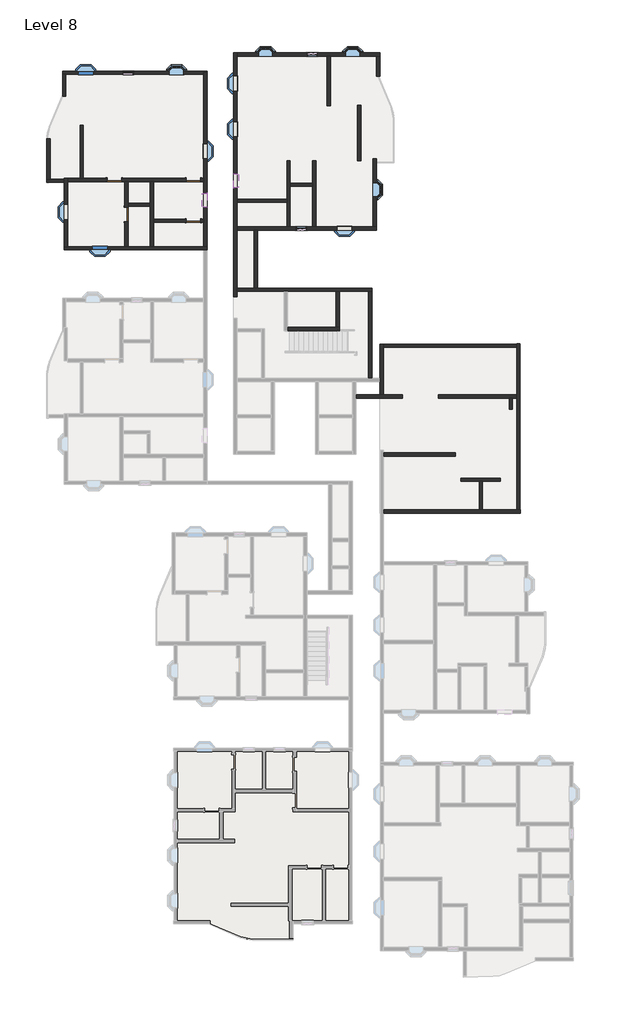
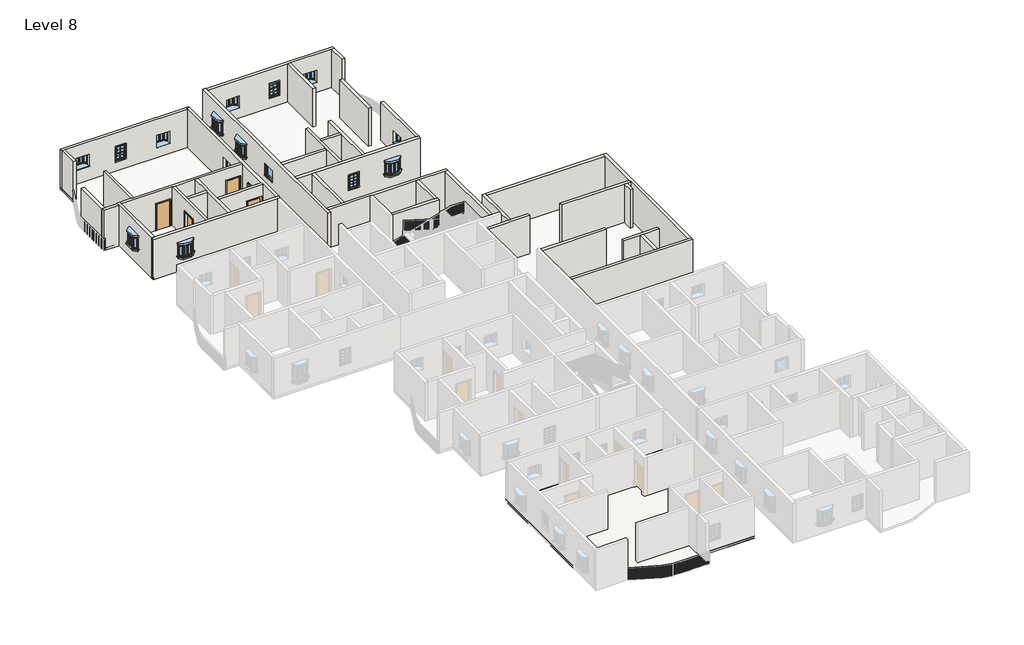
# One storey, part 4 of 14: 39 walls, 16 windows, 4 doors, 2 roofs.
"""IFC4 building model written with IfcOpenShell, lengths in millimetres."""

from ifc_helpers import new_model, si_unit, point, frame, frame_2d, origin, place, context, project, spatial, polyline, circle_curve, trimmed, segment, composite_curve, outline, extrude, faceted_brep, transform, mapped, element, save
from components import door_719f80de, window_910x910mm_67ef725a, window_8debb0fa, windows_sgl_w_glazing_bars_910x910mm_256712d0

model = new_model("IFC4")

# Units and contexts
model_context = context("Model", 3, world=origin())
ifc_project = project(units=[si_unit("LENGTHUNIT", "METRE", prefix="MILLI")], contexts=[model_context])

# Site, building, storey
site = spatial("IfcSite", under=ifc_project)
building = spatial("IfcBuilding", under=site)
storey = spatial("IfcBuildingStorey", under=building, Name="Level 8", Elevation=21336.0)

# Doors
placement = place(None, origin())
door_shape = door_719f80de(model_context)
element("IfcDoor", 1, ObjectType="Single-Flush : 36\" x 84\"", at=placement, inside=storey, context=model_context, shape_type="MappedRepresentation", body=[
    mapped(door_shape, transform((-16068.1391351, 22048.4083494, 21336.0), x_axis=(1.0, 0.0, 0.0), y_axis=(0.0, 1.0, 0.0), z_axis=(0.0, 0.0, 1.0))),
])
element("IfcDoor", 2, ObjectType="Single-Flush : 36\" x 84\"", at=placement, inside=storey, context=model_context, shape_type="MappedRepresentation", body=[
    mapped(door_shape, transform((-15306.1391351, 19864.0083494, 21336.0), x_axis=(0.0, 1.0, 0.0), y_axis=(-1.0, 0.0, 0.0), z_axis=(0.0, 0.0, 1.0))),
])
element("IfcDoor", 3, ObjectType="Single-Flush : 36\" x 84\"", at=placement, inside=storey, context=model_context, shape_type="MappedRepresentation", body=[
    mapped(door_shape, transform((-11057.9891351, 19470.3083494, 21336.0), x_axis=(1.0, 0.0, 0.0), y_axis=(0.0, 1.0, 0.0), z_axis=(0.0, 0.0, 1.0))),
])
element("IfcDoor", 4, ObjectType="Single-Flush : 36\" x 84\"", at=placement, inside=storey, context=model_context, shape_type="MappedRepresentation", body=[
    mapped(door_shape, transform((-11057.9891351, 22048.4083494, 21336.0), x_axis=(1.0, 0.0, 0.0), y_axis=(0.0, 1.0, 0.0), z_axis=(0.0, 0.0, 1.0))),
])

# Roofs
element("IfcRoof", 5, ObjectType="Generic - 12\"", at=placement, inside=storey, context=model_context, shape_type="SweptSolid", body=[
    extrude(outline(composite_curve([segment(polyline([(-10024.8708389, -25100.3416506), (-12290.487215, -25100.3416506), (-12290.487215, -13962.4416506), (-986.8891351, -13962.4416506), (-986.8891351, -25100.3416506), (-4746.0891351, -25100.3416506), (-4746.0891351, -26090.9416506), (-7315.6413127, -26090.9416506)]), True, "CONTINUOUS"), segment(trimmed(circle_curve(frame_2d((-7315.6413127, -24160.5416506)), 1930.4), [point((-7315.6413127, -26090.9416506))], [point((-8075.5356374, -25935.0851906))], False, "CARTESIAN"), True, "CONTINUOUS"), segment(polyline([(-8075.5356374, -25935.0851906), (-10024.8708389, -25100.3416506)]), True, "CONTINUOUS")], self_intersect=False)), frame((0.0, 0.0, 21336.0), z_axis=(0.0, 0.0, 1.0), x_axis=(1.0, 0.0, 0.0)), (0.0, 0.0, 1.0), 152.4),
])
element("IfcRoof", 6, ObjectType="Generic - 12\"", at=placement, inside=storey, context=model_context, shape_type="SweptSolid", body=[
    extrude(outline(composite_curve([segment(polyline([(-10024.8708389, -25100.3416506), (-12290.487215, -25100.3416506), (-12290.487215, -13962.4416506), (-986.8891351, -13962.4416506), (-986.8891351, -25100.3416506), (-4746.0891351, -25100.3416506), (-4746.0891351, -26090.9416506), (-7315.6413127, -26090.9416506)]), True, "CONTINUOUS"), segment(trimmed(circle_curve(frame_2d((-7315.6413127, -24160.5416506)), 1930.4), [point((-7315.6413127, -26090.9416506))], [point((-8075.5356374, -25935.0851906))], False, "CARTESIAN"), True, "CONTINUOUS"), segment(polyline([(-8075.5356374, -25935.0851906), (-10024.8708389, -25100.3416506)]), True, "CONTINUOUS")], self_intersect=False)), frame((0.0, 0.0, 21336.0), z_axis=(0.0, 0.0, 1.0), x_axis=(1.0, 0.0, 0.0)), (0.0, 0.0, 1.0), 152.4),
])

# Walls
element("IfcWall", 7, ObjectType="4.5\" p", at=placement, inside=storey, context=model_context, shape_type="Brep", body=[
    faceted_brep([(-10600.7891351, 21946.8083494, 23469.6), (-10600.7891351, 21946.8083494, 21336.0), (-10397.5891351, 21946.8083494, 21336.0), (-10397.5891351, 21946.8083494, 24384.0), (-13578.9391351, 21946.8083494, 24384.0), (-13782.1391351, 21946.8083494, 24384.0), (-15204.5391351, 21946.8083494, 24384.0), (-15407.7391351, 21946.8083494, 24384.0), (-19033.5891351, 21946.8083494, 24384.0), (-19033.5891351, 21946.8083494, 21336.0), (-16525.3391351, 21946.8083494, 21336.0), (-16525.3391351, 21946.8083494, 23469.6), (-15610.9391351, 21946.8083494, 23469.6), (-15610.9391351, 21946.8083494, 21336.0), (-15407.7391351, 21946.8083494, 21336.0), (-15204.5391351, 21946.8083494, 21336.0), (-13782.1391351, 21946.8083494, 21336.0), (-13578.9391351, 21946.8083494, 21336.0), (-11515.1891351, 21946.8083494, 21336.0), (-11515.1891351, 21946.8083494, 23469.6), (-10397.5891351, 22150.0083494, 21336.0), (-10600.7891351, 22150.0083494, 21336.0), (-10600.7891351, 22150.0083494, 23469.6), (-11515.1891351, 22150.0083494, 23469.6), (-11515.1891351, 22150.0083494, 21336.0), (-15610.9391351, 22150.0083494, 21336.0), (-15610.9391351, 22150.0083494, 23469.6), (-16525.3391351, 22150.0083494, 23469.6), (-16525.3391351, 22150.0083494, 21336.0), (-18042.9891351, 22150.0083494, 21336.0), (-18246.1891351, 22150.0083494, 21336.0), (-19033.5891351, 22150.0083494, 21336.0), (-19033.5891351, 22150.0083494, 24384.0), (-18246.1891351, 22150.0083494, 24384.0), (-18042.9891351, 22150.0083494, 24384.0), (-10397.5891351, 22150.0083494, 24384.0)], [[[0, 1, 2, 3, 4, 5, 6, 7, 8, 9, 10, 11, 12, 13, 14, 15, 16, 17, 18, 19]], [[20, 21, 22, 23, 24, 25, 26, 27, 28, 29, 30, 31, 32, 33, 34, 35]], [[10, 9, 31, 30, 29, 28]], [[2, 1, 21, 20]], [[18, 17, 16, 15, 14, 13, 25, 24]], [[8, 7, 6, 5, 4, 3, 35, 34, 33, 32]], [[9, 8, 32, 31]], [[3, 2, 20, 35]], [[26, 25, 13, 12]], [[27, 26, 12, 11]], [[28, 27, 11, 10]], [[22, 21, 1, 0]], [[23, 22, 0, 19]], [[24, 23, 19, 18]]]),
])
element("IfcWall", 8, ObjectType="4.5\" p", at=placement, inside=storey, context=model_context, shape_type="Brep", body=[
    faceted_brep([(-15407.7391351, 21946.8083494, 21336.0), (-15407.7391351, 20321.2083494, 21336.0), (-15407.7391351, 20321.2083494, 23469.6), (-15407.7391351, 19406.8083494, 23469.6), (-15407.7391351, 19406.8083494, 21336.0), (-15407.7391351, 17812.9583494, 21336.0), (-15407.7391351, 17812.9583494, 24384.0), (-15407.7391351, 21946.8083494, 24384.0), (-15204.5391351, 20321.2083494, 23469.6), (-15204.5391351, 20321.2083494, 21336.0), (-15204.5391351, 20372.0083494, 21336.0), (-15204.5391351, 20575.2083494, 21336.0), (-15204.5391351, 21946.8083494, 21336.0), (-15204.5391351, 21946.8083494, 24384.0), (-15204.5391351, 20575.2083494, 24384.0), (-15204.5391351, 20372.0083494, 24384.0), (-15204.5391351, 17812.9583494, 24384.0), (-15204.5391351, 17812.9583494, 21336.0), (-15204.5391351, 19406.8083494, 21336.0), (-15204.5391351, 19406.8083494, 23469.6)], [[[0, 1, 2, 3, 4, 5, 6, 7]], [[8, 9, 10, 11, 12, 13, 14, 15, 16, 17, 18, 19]], [[18, 17, 5, 4]], [[12, 11, 10, 9, 1, 0]], [[7, 6, 16, 15, 14, 13]], [[6, 5, 17, 16]], [[0, 7, 13, 12]], [[2, 1, 9, 8]], [[3, 2, 8, 19]], [[4, 3, 19, 18]]]),
])
element("IfcWall", 9, ObjectType="4.5\" p", at=placement, inside=storey, context=model_context, shape_type="Brep", body=[
    faceted_brep([(-13782.1391351, 21946.8083494, 21336.0), (-13782.1391351, 20575.2083494, 21336.0), (-13782.1391351, 20372.0083494, 21336.0), (-13782.1391351, 17812.9583494, 21336.0), (-13782.1391351, 17812.9583494, 24384.0), (-13782.1391351, 20372.0083494, 24384.0), (-13782.1391351, 20575.2083494, 24384.0), (-13782.1391351, 21946.8083494, 24384.0), (-13578.9391351, 21946.8083494, 21336.0), (-13578.9391351, 21946.8083494, 24384.0), (-13578.9391351, 19571.9083494, 24384.0), (-13578.9391351, 19368.7083494, 24384.0), (-13578.9391351, 17812.9583494, 24384.0), (-13578.9391351, 17812.9583494, 21336.0), (-13578.9391351, 19368.7083494, 21336.0), (-13578.9391351, 19571.9083494, 21336.0)], [[[0, 1, 2, 3, 4, 5, 6, 7]], [[8, 9, 10, 11, 12, 13, 14, 15]], [[3, 2, 1, 0, 8, 15, 14, 13]], [[7, 6, 5, 4, 12, 11, 10, 9]], [[4, 3, 13, 12]], [[0, 7, 9, 8]]]),
])
element("IfcWall", 10, ObjectType="4.5\" p", at=placement, inside=storey, context=model_context, shape_type="SweptSolid", body=[
    extrude(outline(polyline([(-13782.1391351, 20372.0083494), (-15204.5391351, 20372.0083494), (-15204.5391351, 20575.2083494), (-13782.1391351, 20575.2083494), (-13782.1391351, 20372.0083494)])), frame((0.0, 0.0, 21336.0), z_axis=(0.0, 0.0, 1.0), x_axis=(1.0, 0.0, 0.0)), (0.0, 0.0, 1.0), 3048.0),
])
element("IfcWall", 11, ObjectType="4.5\" p", at=placement, inside=storey, context=model_context, shape_type="SweptSolid", body=[
    extrude(outline(polyline([(23469.6, -10600.7891351), (21336.0, -10600.7891351), (21336.0, -10397.5891351), (24384.0, -10397.5891351), (24384.0, -13578.9391351), (21336.0, -13578.9391351), (21336.0, -11515.1891351), (23469.6, -11515.1891351), (23469.6, -10600.7891351)])), frame((0.0, 19368.7083494, 0.0), z_axis=(0.0, 1.0, 0.0), x_axis=(0.0, 0.0, 1.0)), (0.0, 0.0, 1.0), 203.2),
])
element("IfcWall", 12, ObjectType="4.5\" p", at=placement, inside=storey, context=model_context, shape_type="SweptSolid", body=[
    extrude(outline(polyline([(-18246.1891351, 22150.0083494), (-18246.1891351, 25515.5083494), (-18042.9891351, 25515.5083494), (-18042.9891351, 22150.0083494), (-18246.1891351, 22150.0083494)])), frame((0.0, 0.0, 21336.0), z_axis=(0.0, 0.0, 1.0), x_axis=(1.0, 0.0, 0.0)), (0.0, 0.0, 1.0), 3048.0),
])
element("IfcWall", 13, ObjectType="4.5\" p", at=placement, inside=storey, context=model_context, shape_type="SweptSolid", body=[
    extrude(outline(polyline([(-6993.9891351, 18875.1215905), (-6993.9891351, 15192.1215905), (-7197.1891351, 15192.1215905), (-7197.1891351, 18875.1215905), (-6993.9891351, 18875.1215905)])), frame((0.0, 0.0, 21336.0), z_axis=(0.0, 0.0, 1.0), x_axis=(1.0, 0.0, 0.0)), (0.0, 0.0, 1.0), 3048.0),
])
element("IfcWall", 14, ObjectType="4.5\" p", at=placement, inside=storey, context=model_context, shape_type="Brep", body=[
    faceted_brep([(-8289.3891351, 18875.1215905, 21336.0), (-7197.1891351, 18875.1215905, 21336.0), (-6993.9891351, 18875.1215905, 21336.0), (562.5108649, 18875.1215905, 21336.0), (562.5108649, 18875.1215905, 24384.0), (-6993.9891351, 18875.1215905, 24384.0), (-7197.1891351, 18875.1215905, 24384.0), (-8289.3891351, 18875.1215905, 24384.0), (-1017.6641351, 18875.1215905, 23446.0), (-1017.6641351, 18875.1215905, 22536.0), (-1927.6641351, 18875.1215905, 22536.0), (-1927.6641351, 18875.1215905, 23446.0), (-3876.1391351, 18875.1215905, 23317.2), (-3876.1391351, 18875.1215905, 22250.4), (-4536.5391351, 18875.1215905, 22250.4), (-4536.5391351, 18875.1215905, 23317.2), (-8289.3891351, 19078.3215905, 21336.0), (-8289.3891351, 19078.3215905, 24384.0), (-5120.7391351, 19078.3215905, 24384.0), (-4917.5391351, 19078.3215905, 24384.0), (-3495.1391351, 19078.3215905, 24384.0), (-3291.9391351, 19078.3215905, 24384.0), (346.6108649, 19078.3215905, 24384.0), (549.8108649, 19078.3215905, 24384.0), (562.5108649, 19078.3215905, 24384.0), (562.5108649, 19078.3215905, 21336.0), (549.8108649, 19078.3215905, 21336.0), (346.6108649, 19078.3215905, 21336.0), (-3291.9391351, 19078.3215905, 21336.0), (-3495.1391351, 19078.3215905, 21336.0), (-4917.5391351, 19078.3215905, 21336.0), (-5120.7391351, 19078.3215905, 21336.0), (-1017.6641351, 19078.3215905, 23446.0), (-1927.6641351, 19078.3215905, 23446.0), (-1927.6641351, 19078.3215905, 22536.0), (-1017.6641351, 19078.3215905, 22536.0), (-3876.1391351, 19078.3215905, 23317.2), (-4536.5391351, 19078.3215905, 23317.2), (-4536.5391351, 19078.3215905, 22250.4), (-3876.1391351, 19078.3215905, 22250.4)], [[[0, 1, 2, 3, 4, 5, 6, 7], [8, 9, 10, 11], [12, 13, 14, 15]], [[16, 17, 18, 19, 20, 21, 22, 23, 24, 25, 26, 27, 28, 29, 30, 31], [32, 33, 34, 35], [36, 37, 38, 39]], [[3, 2, 1, 0, 16, 31, 30, 29, 28, 27, 26, 25]], [[4, 3, 25, 24]], [[7, 6, 5, 4, 24, 23, 22, 21, 20, 19, 18, 17]], [[0, 7, 17, 16]], [[9, 8, 32, 35]], [[10, 9, 35, 34]], [[11, 10, 34, 33]], [[8, 11, 33, 32]], [[13, 12, 36, 39]], [[14, 13, 39, 38]], [[15, 14, 38, 37]], [[12, 15, 37, 36]]]),
])
element("IfcWall", 15, ObjectType="4.5\" p", at=placement, inside=storey, context=model_context, shape_type="SweptSolid", body=[
    extrude(outline(polyline([(19078.3215905, 21336.0), (19078.3215905, 24384.0), (23396.3215905, 24384.0), (23396.3215905, 21336.0), (19078.3215905, 21336.0)]), holes=[polyline([(21882.8215905, 23160.4), (20972.8215905, 23160.4), (20972.8215905, 22250.4), (21882.8215905, 22250.4), (21882.8215905, 23160.4)])]), frame((346.6108649, 0.0, 0.0), z_axis=(1.0, 0.0, 0.0), x_axis=(0.0, 1.0, 0.0)), (0.0, 0.0, 1.0), 203.2),
])
element("IfcWall", 16, ObjectType="4.5\" p", at=placement, inside=storey, context=model_context, shape_type="SweptSolid", body=[
    extrude(outline(polyline([(-5120.7391351, 20634.0715905), (-8289.3891351, 20634.0715905), (-8289.3891351, 20837.2715905), (-5120.7391351, 20837.2715905), (-5120.7391351, 20634.0715905)])), frame((0.0, 0.0, 21336.0), z_axis=(0.0, 0.0, 1.0), x_axis=(1.0, 0.0, 0.0)), (0.0, 0.0, 1.0), 3048.0),
])
element("IfcWall", 17, ObjectType="4.5\" p", at=placement, inside=storey, context=model_context, shape_type="Brep", body=[
    faceted_brep([(-5120.7391351, 23256.6215905, 21336.0), (-5120.7391351, 20837.2715905, 21336.0), (-5120.7391351, 20634.0715905, 21336.0), (-5120.7391351, 19078.3215905, 21336.0), (-5120.7391351, 19078.3215905, 24384.0), (-5120.7391351, 20634.0715905, 24384.0), (-5120.7391351, 20837.2715905, 24384.0), (-5120.7391351, 23256.6215905, 24384.0), (-4917.5391351, 23256.6215905, 21336.0), (-4917.5391351, 23256.6215905, 24384.0), (-4917.5391351, 21853.2715905, 24384.0), (-4917.5391351, 21650.0715905, 24384.0), (-4917.5391351, 19078.3215905, 24384.0), (-4917.5391351, 19078.3215905, 21336.0), (-4917.5391351, 21650.0715905, 21336.0), (-4917.5391351, 21853.2715905, 21336.0)], [[[0, 1, 2, 3, 4, 5, 6, 7]], [[8, 9, 10, 11, 12, 13, 14, 15]], [[3, 2, 1, 0, 8, 15, 14, 13]], [[7, 6, 5, 4, 12, 11, 10, 9]], [[0, 7, 9, 8]], [[4, 3, 13, 12]]]),
])
element("IfcWall", 18, ObjectType="4.5\" p", at=placement, inside=storey, context=model_context, shape_type="Brep", body=[
    faceted_brep([(-3495.1391351, 23256.6215905, 21336.0), (-3495.1391351, 21853.2715905, 21336.0), (-3495.1391351, 21650.0715905, 21336.0), (-3495.1391351, 19078.3215905, 21336.0), (-3495.1391351, 19078.3215905, 24384.0), (-3495.1391351, 21650.0715905, 24384.0), (-3495.1391351, 21853.2715905, 24384.0), (-3495.1391351, 23256.6215905, 24384.0), (-3291.9391351, 23256.6215905, 21336.0), (-3291.9391351, 23256.6215905, 24384.0), (-3291.9391351, 19078.3215905, 24384.0), (-3291.9391351, 19078.3215905, 21336.0)], [[[0, 1, 2, 3, 4, 5, 6, 7]], [[8, 9, 10, 11]], [[3, 2, 1, 0, 8, 11]], [[7, 6, 5, 4, 10, 9]], [[0, 7, 9, 8]], [[4, 3, 11, 10]]]),
])
element("IfcWall", 19, ObjectType="4.5\" p", at=placement, inside=storey, context=model_context, shape_type="SweptSolid", body=[
    extrude(outline(polyline([(-3495.1391351, 21650.0715905), (-4917.5391351, 21650.0715905), (-4917.5391351, 21853.2715905), (-3495.1391351, 21853.2715905), (-3495.1391351, 21650.0715905)])), frame((0.0, 0.0, 21336.0), z_axis=(0.0, 0.0, 1.0), x_axis=(1.0, 0.0, 0.0)), (0.0, 0.0, 1.0), 3048.0),
])
element("IfcWall", 20, ObjectType="4.5\" p", at=placement, inside=storey, context=model_context, shape_type="SweptSolid", body=[
    extrude(outline(polyline([(-1799.6891351, 14988.9215905), (-1799.6891351, 12709.2715905), (-2002.8891351, 12709.2715905), (-2002.8891351, 14988.9215905), (-1799.6891351, 14988.9215905)])), frame((0.0, 0.0, 21336.0), z_axis=(0.0, 0.0, 1.0), x_axis=(1.0, 0.0, 0.0)), (0.0, 0.0, 1.0), 3048.0),
])
element("IfcWall", 21, ObjectType="4.5\" p", at=placement, inside=storey, context=model_context, shape_type="Brep", body=[
    faceted_brep([(-5095.3391351, 12506.0715905, 21336.0), (-1786.9891351, 12506.0715905, 21336.0), (-1786.9891351, 12506.0715905, 24384.0), (-5095.3391351, 12506.0715905, 24384.0), (-5095.3391351, 12709.2715905, 21336.0), (-5095.3391351, 12709.2715905, 24384.0), (-2002.8891351, 12709.2715905, 24384.0), (-1799.6891351, 12709.2715905, 24384.0), (-1786.9891351, 12709.2715905, 24384.0), (-1786.9891351, 12709.2715905, 21336.0), (-1799.6891351, 12709.2715905, 21336.0), (-2002.8891351, 12709.2715905, 21336.0)], [[[0, 1, 2, 3]], [[4, 5, 6, 7, 8, 9, 10, 11]], [[1, 0, 4, 11, 10, 9]], [[2, 1, 9, 8]], [[3, 2, 8, 7, 6, 5]], [[0, 3, 5, 4]]]),
])
element("IfcWall", 22, ObjectType="4.5\" p", at=placement, inside=storey, context=model_context, shape_type="Brep", body=[
    faceted_brep([(-745.5891351, 8223.6457306, 21336.0), (2209.4205024, 8223.6457306, 21336.0), (2209.4205024, 8223.6457306, 24384.0), (-745.5891351, 8223.6457306, 24384.0), (-745.5891351, 8426.8457306, 21336.0), (-745.5891351, 8426.8457306, 24384.0), (793.5880523, 8426.8457306, 24384.0), (996.7880523, 8426.8457306, 24384.0), (2209.4205024, 8426.8457306, 24384.0), (2209.4205024, 8426.8457306, 21336.0), (996.7880523, 8426.8457306, 21336.0), (793.5880523, 8426.8457306, 21336.0)], [[[0, 1, 2, 3]], [[4, 5, 6, 7, 8, 9, 10, 11]], [[1, 0, 4, 11, 10, 9]], [[2, 1, 9, 8]], [[3, 2, 8, 7, 6, 5]], [[0, 3, 5, 4]]]),
])
element("IfcWall", 23, ObjectType="4.5\" p", at=placement, inside=storey, context=model_context, shape_type="Brep", body=[
    faceted_brep([(996.7880523, 8426.8457306, 21336.0), (996.7880523, 11443.0957306, 21336.0), (996.7880523, 11646.2957306, 21336.0), (996.7880523, 11646.2957306, 24384.0), (996.7880523, 11443.0957306, 24384.0), (996.7880523, 8426.8457306, 24384.0), (793.5880523, 8426.8457306, 21336.0), (793.5880523, 8426.8457306, 24384.0), (793.5880523, 9275.2949943, 24384.0), (793.5880523, 9478.4949943, 24384.0), (793.5880523, 11646.2957306, 24384.0), (793.5880523, 11646.2957306, 21336.0), (793.5880523, 9478.4949943, 21336.0), (793.5880523, 9275.2949943, 21336.0)], [[[0, 1, 2, 3, 4, 5]], [[6, 7, 8, 9, 10, 11, 12, 13]], [[2, 1, 0, 6, 13, 12, 11]], [[5, 4, 3, 10, 9, 8, 7]], [[0, 5, 7, 6]], [[3, 2, 11, 10]]]),
])
element("IfcWall", 24, ObjectType="4.5\" p", at=placement, inside=storey, context=model_context, shape_type="Brep", body=[
    faceted_brep([(9461.3380523, 8426.8457306, 21336.0), (4492.3034266, 8426.8457306, 21336.0), (4492.3034266, 8426.8457306, 24384.0), (9461.3380523, 8426.8457306, 24384.0), (9461.3380523, 8223.6457306, 21336.0), (9461.3380523, 8223.6457306, 24384.0), (9181.9380523, 8223.6457306, 24384.0), (8978.7380523, 8223.6457306, 24384.0), (4492.3034266, 8223.6457306, 24384.0), (4492.3034266, 8223.6457306, 21336.0), (8978.7380523, 8223.6457306, 21336.0), (9181.9380523, 8223.6457306, 21336.0)], [[[0, 1, 2, 3]], [[4, 5, 6, 7, 8, 9, 10, 11]], [[1, 0, 4, 11, 10, 9]], [[2, 1, 9, 8]], [[3, 2, 8, 7, 6, 5]], [[0, 3, 5, 4]]]),
])
element("IfcWall", 25, ObjectType="4.5\" p", at=placement, inside=storey, context=model_context, shape_type="Brep", body=[
    faceted_brep([(1007.0108649, 940.1957306, 21336.0), (9677.2380523, 940.1957306, 21336.0), (9677.2380523, 940.1957306, 24384.0), (1007.0108649, 940.1957306, 24384.0), (1007.0108649, 1143.3957306, 21336.0), (1007.0108649, 1143.3957306, 24384.0), (7073.7380523, 1143.3957306, 24384.0), (7276.9380523, 1143.3957306, 24384.0), (9461.3380523, 1143.3957306, 24384.0), (9664.5380523, 1143.3957306, 24384.0), (9677.2380523, 1143.3957306, 24384.0), (9677.2380523, 1143.3957306, 21336.0), (9664.5380523, 1143.3957306, 21336.0), (9461.3380523, 1143.3957306, 21336.0), (7276.9380523, 1143.3957306, 21336.0), (7073.7380523, 1143.3957306, 21336.0)], [[[0, 1, 2, 3]], [[4, 5, 6, 7, 8, 9, 10, 11, 12, 13, 14, 15]], [[1, 0, 4, 15, 14, 13, 12, 11]], [[2, 1, 11, 10]], [[3, 2, 10, 9, 8, 7, 6, 5]], [[0, 3, 5, 4]]]),
])
element("IfcWall", 26, ObjectType="4.5\" p", at=placement, inside=storey, context=model_context, shape_type="Brep", body=[
    faceted_brep([(9664.5380523, 1143.3957306, 21336.0), (9664.5380523, 11658.9957306, 21336.0), (9664.5380523, 11658.9957306, 24384.0), (9664.5380523, 1143.3957306, 24384.0), (9461.3380523, 1143.3957306, 21336.0), (9461.3380523, 1143.3957306, 24384.0), (9461.3380523, 8223.6457306, 24384.0), (9461.3380523, 8426.8457306, 24384.0), (9461.3380523, 11443.0957306, 24384.0), (9461.3380523, 11646.2957306, 24384.0), (9461.3380523, 11658.9957306, 24384.0), (9461.3380523, 11658.9957306, 21336.0), (9461.3380523, 11646.2957306, 21336.0), (9461.3380523, 11443.0957306, 21336.0), (9461.3380523, 8426.8457306, 21336.0), (9461.3380523, 8223.6457306, 21336.0)], [[[0, 1, 2, 3]], [[4, 5, 6, 7, 8, 9, 10, 11, 12, 13, 14, 15]], [[1, 0, 4, 15, 14, 13, 12, 11]], [[2, 1, 11, 10]], [[3, 2, 10, 9, 8, 7, 6, 5]], [[0, 3, 5, 4]]]),
])
element("IfcWall", 27, ObjectType="4.5\" p", at=placement, inside=storey, context=model_context, shape_type="SweptSolid", body=[
    extrude(outline(polyline([(-643.9891351, 23256.6215905), (-643.9891351, 26780.8715905), (-440.7891351, 26780.8715905), (-440.7891351, 23256.6215905), (-643.9891351, 23256.6215905)])), frame((0.0, 0.0, 21336.0), z_axis=(0.0, 0.0, 1.0), x_axis=(1.0, 0.0, 0.0)), (0.0, 0.0, 1.0), 3048.0),
])
element("IfcWall", 28, ObjectType="4.5\" p", at=placement, inside=storey, context=model_context, shape_type="SweptSolid", body=[
    extrude(outline(polyline([(-2568.0391351, 26760.9286213), (-2568.0391351, 29898.7215905), (-2364.8391351, 29898.7215905), (-2364.8391351, 26760.9286213), (-2568.0391351, 26760.9286213)])), frame((0.0, 0.0, 21336.0), z_axis=(0.0, 0.0, 1.0), x_axis=(1.0, 0.0, 0.0)), (0.0, 0.0, 1.0), 3048.0),
])
element("IfcWall", 29, ObjectType="4.5\" p", at=placement, inside=storey, context=model_context, shape_type="SweptSolid", body=[
    extrude(outline(polyline([(765.7108649, 29898.7215905), (765.7108649, 28631.1875845), (562.5108649, 28631.1875845), (562.5108649, 29898.7215905), (765.7108649, 29898.7215905)])), frame((0.0, 0.0, 21336.0), z_axis=(0.0, 0.0, 1.0), x_axis=(1.0, 0.0, 0.0)), (0.0, 0.0, 1.0), 3048.0),
])
element("IfcWall", 30, ObjectType="9\" w", at=placement, inside=storey, context=model_context, shape_type="Brep", body=[
    faceted_brep([(-10181.6891351, 17812.9583494, 21336.0), (-10194.3891351, 17812.9583494, 21336.0), (-10397.5891351, 17812.9583494, 21336.0), (-13578.9391351, 17812.9583494, 21336.0), (-13782.1391351, 17812.9583494, 21336.0), (-15204.5391351, 17812.9583494, 21336.0), (-15407.7391351, 17812.9583494, 21336.0), (-19033.5891351, 17812.9583494, 21336.0), (-19236.7891351, 17812.9583494, 21336.0), (-19249.4891351, 17812.9583494, 21336.0), (-19249.4891351, 17812.9583494, 24384.0), (-19236.7891351, 17812.9583494, 24384.0), (-19033.5891351, 17812.9583494, 24384.0), (-15407.7391351, 17812.9583494, 24384.0), (-15204.5391351, 17812.9583494, 24384.0), (-13782.1391351, 17812.9583494, 24384.0), (-13578.9391351, 17812.9583494, 24384.0), (-10397.5891351, 17812.9583494, 24384.0), (-10194.3891351, 17812.9583494, 24384.0), (-10181.6891351, 17812.9583494, 24384.0), (-16527.5391351, 17812.9583494, 23446.0), (-17437.5391351, 17812.9583494, 23446.0), (-17437.5391351, 17812.9583494, 22536.0), (-16527.5391351, 17812.9583494, 22536.0), (-10181.6891351, 17609.7583494, 21336.0), (-10181.6891351, 17609.7583494, 24384.0), (-19249.4891351, 17609.7583494, 24384.0), (-19249.4891351, 17609.7583494, 21336.0), (-16527.5391351, 17609.7583494, 23446.0), (-16527.5391351, 17609.7583494, 22536.0), (-17437.5391351, 17609.7583494, 22536.0), (-17437.5391351, 17609.7583494, 23446.0)], [[[0, 1, 2, 3, 4, 5, 6, 7, 8, 9, 10, 11, 12, 13, 14, 15, 16, 17, 18, 19], [20, 21, 22, 23]], [[24, 25, 26, 27], [28, 29, 30, 31]], [[9, 8, 7, 6, 5, 4, 3, 2, 1, 0, 24, 27]], [[10, 9, 27, 26]], [[19, 18, 17, 16, 15, 14, 13, 12, 11, 10, 26, 25]], [[0, 19, 25, 24]], [[29, 28, 20, 23]], [[30, 29, 23, 22]], [[31, 30, 22, 21]], [[28, 31, 21, 20]]]),
])
element("IfcWall", 31, ObjectType="9\" w", at=placement, inside=storey, context=model_context, shape_type="Brep", body=[
    faceted_brep([(-19033.5891351, 17812.9583494, 21336.0), (-19033.5891351, 21946.8083494, 21336.0), (-19033.5891351, 22150.0083494, 21336.0), (-19033.5891351, 22150.0083494, 24384.0), (-19033.5891351, 21946.8083494, 24384.0), (-19033.5891351, 17812.9583494, 24384.0), (-19033.5891351, 19555.0583494, 23446.0), (-19033.5891351, 20465.0583494, 23446.0), (-19033.5891351, 20465.0583494, 22536.0), (-19033.5891351, 19555.0583494, 22536.0), (-19236.7891351, 17812.9583494, 21336.0), (-19236.7891351, 17812.9583494, 24384.0), (-19236.7891351, 21889.6583494, 24384.0), (-19236.7891351, 22092.8583494, 24384.0), (-19236.7891351, 22150.0083494, 24384.0), (-19236.7891351, 22150.0083494, 21336.0), (-19236.7891351, 22092.8583494, 21336.0), (-19236.7891351, 21889.6583494, 21336.0), (-19236.7891351, 19555.0583494, 23446.0), (-19236.7891351, 19555.0583494, 22536.0), (-19236.7891351, 20465.0583494, 22536.0), (-19236.7891351, 20465.0583494, 23446.0)], [[[0, 1, 2, 3, 4, 5], [6, 7, 8, 9]], [[10, 11, 12, 13, 14, 15, 16, 17], [18, 19, 20, 21]], [[2, 1, 0, 10, 17, 16, 15]], [[5, 4, 3, 14, 13, 12, 11]], [[0, 5, 11, 10]], [[3, 2, 15, 14]], [[19, 18, 6, 9]], [[20, 19, 9, 8]], [[21, 20, 8, 7]], [[18, 21, 7, 6]]]),
])
element("IfcWall", 32, ObjectType="9\" w", at=placement, inside=storey, context=model_context, shape_type="Brep", body=[
    faceted_brep([(-10194.3891351, 17812.9583494, 21336.0), (-10194.3891351, 28849.2583494, 21336.0), (-10194.3891351, 28849.2583494, 24384.0), (-10194.3891351, 17812.9583494, 24384.0), (-10194.3891351, 24319.5083494, 23446.0), (-10194.3891351, 24319.5083494, 22536.0), (-10194.3891351, 23409.5083494, 22536.0), (-10194.3891351, 23409.5083494, 23446.0), (-10194.3891351, 20304.3583494, 23446.0), (-10194.3891351, 21214.3583494, 23446.0), (-10194.3891351, 21214.3583494, 22536.0), (-10194.3891351, 20304.3583494, 22536.0), (-10397.5891351, 17812.9583494, 21336.0), (-10397.5891351, 17812.9583494, 24384.0), (-10397.5891351, 19368.7083494, 24384.0), (-10397.5891351, 19571.9083494, 24384.0), (-10397.5891351, 21946.8083494, 24384.0), (-10397.5891351, 22150.0083494, 24384.0), (-10397.5891351, 28849.2583494, 24384.0), (-10397.5891351, 28849.2583494, 21336.0), (-10397.5891351, 22150.0083494, 21336.0), (-10397.5891351, 21946.8083494, 21336.0), (-10397.5891351, 19571.9083494, 21336.0), (-10397.5891351, 19368.7083494, 21336.0), (-10397.5891351, 24319.5083494, 23446.0), (-10397.5891351, 23409.5083494, 23446.0), (-10397.5891351, 23409.5083494, 22536.0), (-10397.5891351, 24319.5083494, 22536.0), (-10397.5891351, 20304.3583494, 23446.0), (-10397.5891351, 20304.3583494, 22536.0), (-10397.5891351, 21214.3583494, 22536.0), (-10397.5891351, 21214.3583494, 23446.0)], [[[0, 1, 2, 3], [4, 5, 6, 7], [8, 9, 10, 11]], [[12, 13, 14, 15, 16, 17, 18, 19, 20, 21, 22, 23], [24, 25, 26, 27], [28, 29, 30, 31]], [[1, 0, 12, 23, 22, 21, 20, 19]], [[2, 1, 19, 18]], [[3, 2, 18, 17, 16, 15, 14, 13]], [[0, 3, 13, 12]], [[5, 4, 24, 27]], [[6, 5, 27, 26]], [[7, 6, 26, 25]], [[4, 7, 25, 24]], [[29, 28, 8, 11]], [[30, 29, 11, 10]], [[31, 30, 10, 9]], [[28, 31, 9, 8]]]),
])
element("IfcWall", 33, ObjectType="9\" w", at=placement, inside=storey, context=model_context, shape_type="Brep", body=[
    faceted_brep([(-20341.6891351, 21889.6583494, 21336.0), (-19236.7891351, 21889.6583494, 21336.0), (-19236.7891351, 21889.6583494, 24384.0), (-20341.6891351, 21889.6583494, 24384.0), (-20341.6891351, 22092.8583494, 21336.0), (-20341.6891351, 22092.8583494, 24384.0), (-20138.4891351, 22092.8583494, 24384.0), (-19236.7891351, 22092.8583494, 24384.0), (-19236.7891351, 22092.8583494, 21336.0), (-20138.4891351, 22092.8583494, 21336.0)], [[[0, 1, 2, 3]], [[4, 5, 6, 7, 8, 9]], [[1, 0, 4, 9, 8]], [[3, 2, 7, 6, 5]], [[0, 3, 5, 4]], [[2, 1, 8, 7]]]),
])
element("IfcWall", 34, ObjectType="9\" w", at=placement, inside=storey, context=model_context, shape_type="SweptSolid", body=[
    extrude(outline(polyline([(-20341.6891351, 22092.8583494), (-20341.6891351, 24656.5948172), (-20138.4891351, 24656.5948172), (-20138.4891351, 22092.8583494), (-20341.6891351, 22092.8583494)])), frame((0.0, 0.0, 21336.0), z_axis=(0.0, 0.0, 1.0), x_axis=(1.0, 0.0, 0.0)), (0.0, 0.0, 1.0), 3048.0),
])
element("IfcWall", 35, ObjectType="9\" w", at=placement, inside=storey, context=model_context, shape_type="Brep", body=[
    faceted_brep([(-8492.5891351, 30114.6215905, 21336.0), (-8492.5891351, 14654.9471999, 21336.0), (-8492.5891351, 14654.9471999, 24384.0), (-8492.5891351, 30114.6215905, 24384.0), (-8492.5891351, 27703.9922564, 23446.0), (-8492.5891351, 27703.9922564, 22536.0), (-8492.5891351, 28613.9922564, 22536.0), (-8492.5891351, 28613.9922564, 23446.0), (-8492.5891351, 24808.3922564, 23446.0), (-8492.5891351, 24808.3922564, 22536.0), (-8492.5891351, 25718.3922564, 22536.0), (-8492.5891351, 25718.3922564, 23446.0), (-8492.5891351, 22451.1465905, 23446.0), (-8492.5891351, 21541.1465905, 23446.0), (-8492.5891351, 21541.1465905, 22536.0), (-8492.5891351, 22451.1465905, 22536.0), (-8289.3891351, 30114.6215905, 21336.0), (-8289.3891351, 30114.6215905, 24384.0), (-8289.3891351, 30101.9215905, 24384.0), (-8289.3891351, 29898.7215905, 24384.0), (-8289.3891351, 20837.2715905, 24384.0), (-8289.3891351, 20634.0715905, 24384.0), (-8289.3891351, 19078.3215905, 24384.0), (-8289.3891351, 18875.1215905, 24384.0), (-8289.3891351, 15192.1215905, 24384.0), (-8289.3891351, 14988.9215905, 24384.0), (-8289.3891351, 14654.9471999, 24384.0), (-8289.3891351, 14654.9471999, 21336.0), (-8289.3891351, 14988.9215905, 21336.0), (-8289.3891351, 15192.1215905, 21336.0), (-8289.3891351, 18875.1215905, 21336.0), (-8289.3891351, 19078.3215905, 21336.0), (-8289.3891351, 20634.0715905, 21336.0), (-8289.3891351, 20837.2715905, 21336.0), (-8289.3891351, 29898.7215905, 21336.0), (-8289.3891351, 30101.9215905, 21336.0), (-8289.3891351, 27703.9922564, 23446.0), (-8289.3891351, 28613.9922564, 23446.0), (-8289.3891351, 28613.9922564, 22536.0), (-8289.3891351, 27703.9922564, 22536.0), (-8289.3891351, 24808.3922564, 23446.0), (-8289.3891351, 25718.3922564, 23446.0), (-8289.3891351, 25718.3922564, 22536.0), (-8289.3891351, 24808.3922564, 22536.0), (-8289.3891351, 22451.1465905, 23446.0), (-8289.3891351, 22451.1465905, 22536.0), (-8289.3891351, 21541.1465905, 22536.0), (-8289.3891351, 21541.1465905, 23446.0)], [[[0, 1, 2, 3], [4, 5, 6, 7], [8, 9, 10, 11], [12, 13, 14, 15]], [[16, 17, 18, 19, 20, 21, 22, 23, 24, 25, 26, 27, 28, 29, 30, 31, 32, 33, 34, 35], [36, 37, 38, 39], [40, 41, 42, 43], [44, 45, 46, 47]], [[1, 0, 16, 35, 34, 33, 32, 31, 30, 29, 28, 27]], [[2, 1, 27, 26]], [[3, 2, 26, 25, 24, 23, 22, 21, 20, 19, 18, 17]], [[0, 3, 17, 16]], [[5, 4, 36, 39]], [[6, 5, 39, 38]], [[7, 6, 38, 37]], [[4, 7, 37, 36]], [[9, 8, 40, 43]], [[10, 9, 43, 42]], [[11, 10, 42, 41]], [[8, 11, 41, 40]], [[45, 44, 12, 15]], [[46, 45, 15, 14]], [[47, 46, 14, 13]], [[44, 47, 13, 12]]]),
])
element("IfcWall", 36, ObjectType="9\" w", at=placement, inside=storey, context=model_context, shape_type="Brep", body=[
    faceted_brep([(-8289.3891351, 14988.9215905, 21336.0), (-5298.5391351, 14988.9215905, 21336.0), (-5095.3391351, 14988.9215905, 21336.0), (-2002.8891351, 14988.9215905, 21336.0), (-1799.6891351, 14988.9215905, 21336.0), (54.5108649, 14988.9215905, 21336.0), (257.7108649, 14988.9215905, 21336.0), (270.4108649, 14988.9215905, 21336.0), (270.4108649, 14988.9215905, 24384.0), (257.7108649, 14988.9215905, 24384.0), (54.5108649, 14988.9215905, 24384.0), (-1799.6891351, 14988.9215905, 24384.0), (-2002.8891351, 14988.9215905, 24384.0), (-5095.3391351, 14988.9215905, 24384.0), (-5298.5391351, 14988.9215905, 24384.0), (-8289.3891351, 14988.9215905, 24384.0), (-8289.3891351, 15192.1215905, 21336.0), (-8289.3891351, 15192.1215905, 24384.0), (-7197.1891351, 15192.1215905, 24384.0), (-6993.9891351, 15192.1215905, 24384.0), (270.4108649, 15192.1215905, 24384.0), (270.4108649, 15192.1215905, 21336.0), (-6993.9891351, 15192.1215905, 21336.0), (-7197.1891351, 15192.1215905, 21336.0)], [[[0, 1, 2, 3, 4, 5, 6, 7, 8, 9, 10, 11, 12, 13, 14, 15]], [[16, 17, 18, 19, 20, 21, 22, 23]], [[7, 6, 5, 4, 3, 2, 1, 0, 16, 23, 22, 21]], [[8, 7, 21, 20]], [[15, 14, 13, 12, 11, 10, 9, 8, 20, 19, 18, 17]], [[0, 15, 17, 16]]]),
])
element("IfcWall", 37, ObjectType="9\" w", at=placement, inside=storey, context=model_context, shape_type="SweptSolid", body=[
    extrude(outline(polyline([(54.5108649, 9478.4949943), (54.5108649, 14988.9215905), (257.7108649, 14988.9215905), (257.7108649, 9478.4949943), (54.5108649, 9478.4949943)])), frame((0.0, 0.0, 21336.0), z_axis=(0.0, 0.0, 1.0), x_axis=(1.0, 0.0, 0.0)), (0.0, 0.0, 1.0), 3048.0),
])
element("IfcWall", 38, ObjectType="9\" w", at=placement, inside=storey, context=model_context, shape_type="SweptSolid", body=[
    extrude(outline(polyline([(9461.3380523, 11443.0957306), (996.7880523, 11443.0957306), (996.7880523, 11646.2957306), (9461.3380523, 11646.2957306), (9461.3380523, 11443.0957306)])), frame((0.0, 0.0, 21336.0), z_axis=(0.0, 0.0, 1.0), x_axis=(1.0, 0.0, 0.0)), (0.0, 0.0, 1.0), 3048.0),
])
element("IfcWall", 39, ObjectType="9\" w", at=placement, inside=storey, context=model_context, shape_type="SweptSolid", body=[
    extrude(outline(polyline([(8978.7380523, 7506.0957306), (8978.7380523, 8223.6457306), (9181.9380523, 8223.6457306), (9181.9380523, 7506.0957306), (8978.7380523, 7506.0957306)])), frame((0.0, 0.0, 21336.0), z_axis=(0.0, 0.0, 1.0), x_axis=(1.0, 0.0, 0.0)), (0.0, 0.0, 1.0), 3048.0),
])
element("IfcWall", 40, ObjectType="9\" w", at=placement, inside=storey, context=model_context, shape_type="SweptSolid", body=[
    extrude(outline(polyline([(7276.9380523, 2954.8622042), (7276.9380523, 1143.3957306), (7073.7380523, 1143.3957306), (7073.7380523, 2954.8622042), (7276.9380523, 2954.8622042)])), frame((0.0, 0.0, 21336.0), z_axis=(0.0, 0.0, 1.0), x_axis=(1.0, 0.0, 0.0)), (0.0, 0.0, 1.0), 3048.0),
])
element("IfcWall", 41, ObjectType="9\" w", at=placement, inside=storey, context=model_context, shape_type="Brep", body=[
    faceted_brep([(5904.1857655, 2954.8622042, 21336.0), (7073.7380523, 2954.8622042, 21336.0), (7276.9380523, 2954.8622042, 21336.0), (8418.7857655, 2954.8622042, 21336.0), (8418.7857655, 2954.8622042, 24384.0), (7276.9380523, 2954.8622042, 24384.0), (7073.7380523, 2954.8622042, 24384.0), (5904.1857655, 2954.8622042, 24384.0), (5904.1857655, 3158.0622042, 21336.0), (5904.1857655, 3158.0622042, 24384.0), (8418.7857655, 3158.0622042, 24384.0), (8418.7857655, 3158.0622042, 21336.0)], [[[0, 1, 2, 3, 4, 5, 6, 7]], [[8, 9, 10, 11]], [[3, 2, 1, 0, 8, 11]], [[4, 3, 11, 10]], [[7, 6, 5, 4, 10, 9]], [[0, 7, 9, 8]]]),
])
element("IfcWall", 42, ObjectType="9\" w", at=placement, inside=storey, context=model_context, shape_type="SweptSolid", body=[
    extrude(outline(polyline([(5571.3060189, 4550.8949943), (1007.0108649, 4550.8949943), (1007.0108649, 4754.0949943), (5571.3060189, 4754.0949943), (5571.3060189, 4550.8949943)])), frame((0.0, 0.0, 21336.0), z_axis=(0.0, 0.0, 1.0), x_axis=(1.0, 0.0, 0.0)), (0.0, 0.0, 1.0), 3048.0),
])
element("IfcWall", 43, ObjectType="9\" w", at=placement, inside=storey, context=model_context, shape_type="Brep", body=[
    faceted_brep([(-8289.3891351, 29898.7215905, 21336.0), (-2568.0391351, 29898.7215905, 21336.0), (-2364.8391351, 29898.7215905, 21336.0), (562.5108649, 29898.7215905, 21336.0), (765.7108649, 29898.7215905, 21336.0), (765.7108649, 29898.7215905, 24384.0), (562.5108649, 29898.7215905, 24384.0), (-2364.8391351, 29898.7215905, 24384.0), (-2568.0391351, 29898.7215905, 24384.0), (-8289.3891351, 29898.7215905, 24384.0), (-6931.4641351, 29898.7215905, 23160.4), (-6021.4641351, 29898.7215905, 23160.4), (-6021.4641351, 29898.7215905, 22250.4), (-6931.4641351, 29898.7215905, 22250.4), (-1406.9641351, 29898.7215905, 23160.4), (-496.9641351, 29898.7215905, 23160.4), (-496.9641351, 29898.7215905, 22250.4), (-1406.9641351, 29898.7215905, 22250.4), (-3844.3891351, 29898.7215905, 23317.2), (-3183.9891351, 29898.7215905, 23317.2), (-3183.9891351, 29898.7215905, 22250.4), (-3844.3891351, 29898.7215905, 22250.4), (-8289.3891351, 30101.9215905, 21336.0), (-8289.3891351, 30101.9215905, 24384.0), (765.7108649, 30101.9215905, 24384.0), (765.7108649, 30101.9215905, 21336.0), (-6931.4641351, 30101.9215905, 23160.4), (-6931.4641351, 30101.9215905, 22250.4), (-6021.4641351, 30101.9215905, 22250.4), (-6021.4641351, 30101.9215905, 23160.4), (-1406.9641351, 30101.9215905, 23160.4), (-1406.9641351, 30101.9215905, 22250.4), (-496.9641351, 30101.9215905, 22250.4), (-496.9641351, 30101.9215905, 23160.4), (-3844.3891351, 30101.9215905, 23317.2), (-3844.3891351, 30101.9215905, 22250.4), (-3183.9891351, 30101.9215905, 22250.4), (-3183.9891351, 30101.9215905, 23317.2)], [[[0, 1, 2, 3, 4, 5, 6, 7, 8, 9], [10, 11, 12, 13], [14, 15, 16, 17], [18, 19, 20, 21]], [[22, 23, 24, 25], [26, 27, 28, 29], [30, 31, 32, 33], [34, 35, 36, 37]], [[4, 3, 2, 1, 0, 22, 25]], [[9, 8, 7, 6, 5, 24, 23]], [[27, 26, 10, 13]], [[28, 27, 13, 12]], [[29, 28, 12, 11]], [[26, 29, 11, 10]], [[31, 30, 14, 17]], [[32, 31, 17, 16]], [[33, 32, 16, 15]], [[30, 33, 15, 14]], [[35, 34, 18, 21]], [[36, 35, 21, 20]], [[37, 36, 20, 19]], [[34, 37, 19, 18]], [[0, 9, 23, 22]], [[5, 4, 25, 24]]]),
])
element("IfcWall", 44, ObjectType="9\" w", at=placement, inside=storey, context=model_context, shape_type="Brep", body=[
    faceted_brep([(-19351.0891351, 28747.6583494, 21336.0), (-19147.8891351, 28747.6583494, 21336.0), (-10181.6891351, 28747.6583494, 21336.0), (-10181.6891351, 28747.6583494, 24384.0), (-19147.8891351, 28747.6583494, 24384.0), (-19351.0891351, 28747.6583494, 24384.0), (-18332.8891351, 28747.6583494, 23446.0), (-17422.8891351, 28747.6583494, 23446.0), (-17422.8891351, 28747.6583494, 22536.0), (-18332.8891351, 28747.6583494, 22536.0), (-12579.7891351, 28747.6583494, 23160.4), (-11669.7891351, 28747.6583494, 23160.4), (-11669.7891351, 28747.6583494, 22250.4), (-12579.7891351, 28747.6583494, 22250.4), (-14845.7641351, 28747.6583494, 23317.2), (-14845.7641351, 28747.6583494, 22250.4), (-15506.1641351, 28747.6583494, 22250.4), (-15506.1641351, 28747.6583494, 23317.2), (-19351.0891351, 28950.8583494, 21336.0), (-19351.0891351, 28950.8583494, 24384.0), (-10181.6891351, 28950.8583494, 24384.0), (-10181.6891351, 28950.8583494, 21336.0), (-18332.8891351, 28950.8583494, 23446.0), (-18332.8891351, 28950.8583494, 22536.0), (-17422.8891351, 28950.8583494, 22536.0), (-17422.8891351, 28950.8583494, 23446.0), (-12579.7891351, 28950.8583494, 23160.4), (-12579.7891351, 28950.8583494, 22250.4), (-11669.7891351, 28950.8583494, 22250.4), (-11669.7891351, 28950.8583494, 23160.4), (-14845.7641351, 28950.8583494, 23317.2), (-15506.1641351, 28950.8583494, 23317.2), (-15506.1641351, 28950.8583494, 22250.4), (-14845.7641351, 28950.8583494, 22250.4)], [[[0, 1, 2, 3, 4, 5], [6, 7, 8, 9], [10, 11, 12, 13], [14, 15, 16, 17]], [[18, 19, 20, 21], [22, 23, 24, 25], [26, 27, 28, 29], [30, 31, 32, 33]], [[2, 1, 0, 18, 21]], [[3, 2, 21, 20]], [[5, 4, 3, 20, 19]], [[23, 22, 6, 9]], [[24, 23, 9, 8]], [[25, 24, 8, 7]], [[22, 25, 7, 6]], [[27, 26, 10, 13]], [[28, 27, 13, 12]], [[29, 28, 12, 11]], [[26, 29, 11, 10]], [[15, 14, 30, 33]], [[16, 15, 33, 32]], [[17, 16, 32, 31]], [[14, 17, 31, 30]], [[0, 5, 19, 18]]]),
])
element("IfcWall", 45, ObjectType="9\" w", at=placement, inside=storey, context=model_context, shape_type="SweptSolid", body=[
    extrude(outline(polyline([(-19147.8891351, 28747.6583494), (-19147.8891351, 27344.9858981), (-19351.0891351, 27344.9858981), (-19351.0891351, 28747.6583494), (-19147.8891351, 28747.6583494)])), frame((0.0, 0.0, 21336.0), z_axis=(0.0, 0.0, 1.0), x_axis=(1.0, 0.0, 0.0)), (0.0, 0.0, 1.0), 3048.0),
])

# Windows
window_910x910mm_shape = window_910x910mm_67ef725a(model_context)
element("IfcWindow", 46, ObjectType="910x910mm", at=placement, inside=storey, context=model_context, shape_type="MappedRepresentation", body=[
    mapped(window_910x910mm_shape, transform((-10304.445703, 23294.5083494, 21336.0), x_axis=(0.0, -1.0, 0.0), y_axis=(1.0, 0.0, 0.0), z_axis=(0.0, 0.0, 1.0))),
])
element("IfcWindow", 47, ObjectType="910x910mm", at=placement, inside=storey, context=model_context, shape_type="MappedRepresentation", body=[
    mapped(window_910x910mm_shape, transform((-19126.7325673, 20580.0583494, 21336.0), x_axis=(0.0, 1.0, 0.0), y_axis=(-1.0, 0.0, 0.0), z_axis=(0.0, 0.0, 1.0))),
])
element("IfcWindow", 48, ObjectType="910x910mm", at=placement, inside=storey, context=model_context, shape_type="MappedRepresentation", body=[
    mapped(window_910x910mm_shape, transform((-17552.5391351, 17719.8149172, 21336.0), x_axis=(-1.0, 0.0, 0.0), y_axis=(0.0, -1.0, 0.0), z_axis=(0.0, 0.0, 1.0))),
])
element("IfcWindow", 49, ObjectType="910x910mm", at=placement, inside=storey, context=model_context, shape_type="MappedRepresentation", body=[
    mapped(window_910x910mm_shape, transform((-8382.5325673, 28728.9922564, 21336.0), x_axis=(0.0, 1.0, 0.0), y_axis=(-1.0, 0.0, 0.0), z_axis=(0.0, 0.0, 1.0))),
])
element("IfcWindow", 50, ObjectType="910x910mm", at=placement, inside=storey, context=model_context, shape_type="MappedRepresentation", body=[
    mapped(window_910x910mm_shape, transform((-8382.5325673, 25833.3922564, 21336.0), x_axis=(0.0, 1.0, 0.0), y_axis=(-1.0, 0.0, 0.0), z_axis=(0.0, 0.0, 1.0))),
])
element("IfcWindow", 51, ObjectType="910x910mm", at=placement, inside=storey, context=model_context, shape_type="MappedRepresentation", body=[
    mapped(window_910x910mm_shape, transform((-5906.4641351, 29991.8650227, 21050.4), x_axis=(1.0, 0.0, 0.0), y_axis=(0.0, 1.0, 0.0), z_axis=(0.0, 0.0, 1.0))),
])
element("IfcWindow", 52, ObjectType="910x910mm", at=placement, inside=storey, context=model_context, shape_type="MappedRepresentation", body=[
    mapped(window_910x910mm_shape, transform((-381.9641351, 29991.8650227, 21050.4), x_axis=(1.0, 0.0, 0.0), y_axis=(0.0, 1.0, 0.0), z_axis=(0.0, 0.0, 1.0))),
])
element("IfcWindow", 53, ObjectType="910x910mm", at=placement, inside=storey, context=model_context, shape_type="MappedRepresentation", body=[
    mapped(window_910x910mm_shape, transform((-17307.8891351, 28840.8017816, 21336.0), x_axis=(1.0, 0.0, 0.0), y_axis=(0.0, 1.0, 0.0), z_axis=(0.0, 0.0, 1.0))),
])
element("IfcWindow", 54, ObjectType="910x910mm", at=placement, inside=storey, context=model_context, shape_type="MappedRepresentation", body=[
    mapped(window_910x910mm_shape, transform((-11554.7891351, 28840.8017816, 21050.4), x_axis=(1.0, 0.0, 0.0), y_axis=(0.0, 1.0, 0.0), z_axis=(0.0, 0.0, 1.0))),
])
element("IfcWindow", 55, ObjectType="910x910mm", at=placement, inside=storey, context=model_context, shape_type="MappedRepresentation", body=[
    mapped(window_910x910mm_shape, transform((439.754297, 20857.8215905, 21050.4), x_axis=(0.0, -1.0, 0.0), y_axis=(1.0, 0.0, 0.0), z_axis=(0.0, 0.0, 1.0))),
])
element("IfcWindow", 56, ObjectType="910x910mm", at=placement, inside=storey, context=model_context, shape_type="MappedRepresentation", body=[
    mapped(window_910x910mm_shape, transform((-2042.6641351, 18985.1781583, 21336.0), x_axis=(-1.0, 0.0, 0.0), y_axis=(0.0, -1.0, 0.0), z_axis=(0.0, 0.0, 1.0))),
])
window_shape = window_8debb0fa(model_context)
element("IfcWindow", 57, ObjectType="Window-Double-Hung : 26\" x 42\"", at=placement, inside=storey, context=model_context, shape_type="MappedRepresentation", body=[
    mapped(window_shape, transform((-3514.1891351, 30000.3215905, 21336.0), x_axis=(1.0, 0.0, 0.0), y_axis=(0.0, 1.0, 0.0), z_axis=(0.0, 0.0, 1.0))),
])
element("IfcWindow", 58, ObjectType="Window-Double-Hung : 26\" x 42\"", at=placement, inside=storey, context=model_context, shape_type="MappedRepresentation", body=[
    mapped(window_shape, transform((-15175.9641351, 28849.2583494, 21336.0), x_axis=(-1.0, 0.0, 0.0), y_axis=(0.0, -1.0, 0.0), z_axis=(0.0, 0.0, 1.0))),
])
element("IfcWindow", 59, ObjectType="Window-Double-Hung : 26\" x 42\"", at=placement, inside=storey, context=model_context, shape_type="MappedRepresentation", body=[
    mapped(window_shape, transform((-4206.3391351, 18976.7215905, 21336.0), x_axis=(-1.0, 0.0, 0.0), y_axis=(0.0, -1.0, 0.0), z_axis=(0.0, 0.0, 1.0))),
])
windows_sgl_w_glazing_bars_910x910mm_shape = windows_sgl_w_glazing_bars_910x910mm_256712d0(model_context)
element("IfcWindow", 60, ObjectType="Windows_Sgl_w-Glazing_Bars : 910x910mm", at=placement, inside=storey, context=model_context, shape_type="MappedRepresentation", body=[
    mapped(windows_sgl_w_glazing_bars_910x910mm_shape, transform((-10287.5325673, 20759.3583494, 21336.0), x_axis=(0.0, 1.0, 0.0), y_axis=(-1.0, 0.0, 0.0), z_axis=(0.0, 0.0, 1.0))),
])
element("IfcWindow", 61, ObjectType="Windows_Sgl_w-Glazing_Bars : 910x910mm", at=placement, inside=storey, context=model_context, shape_type="MappedRepresentation", body=[
    mapped(windows_sgl_w_glazing_bars_910x910mm_shape, transform((-8399.445703, 21996.1465905, 21336.0), x_axis=(0.0, -1.0, 0.0), y_axis=(1.0, 0.0, 0.0), z_axis=(0.0, 0.0, 1.0))),
])

save(model, "model.ifc")

# Revit data of these elements
# Type "Single-Flush : 36\" x 84\""
#   Type Mark = "1"
#   Construction Type Id = "MDOOR"
#   Assembly Code = "C1020"
#   Analytic Construction = "Metal"
#   Thickness = 0' - 2"
#   Heat Transfer Coefficient (U) = 0.651978 BTU/(h·ft²·°F)
#   Height = 7' - 0"
#   Trim Projection Ext = 0' - 1"
#   Trim Projection Int = 0' - 1"
#   Trim Width = 0' - 3"
#   Width = 3' - 0"
#   Define Thermal Properties by = 1
#   Define Thermal Properties by = 1
#   Door Material = Door - Panel
#   Frame Material = Door - Frame
#   Visual Light Transmittance = 0
#   Solar Heat Gain Coefficient = 0
#   Function = (empty or 0)
#   Wall Closure = (empty or 0)
# Type "Generic - 12\""
#   Assembly Code = "B1020"
#   Layers, outside or top first: 0' - 6" no material (function 1)
# Type "4.5\" p"
#   Assembly Code = "B2010"
#   Layers, outside or top first: 0' - 8" no material (function 1)
# Type "9\" w"
#   Assembly Code = "B2010"
#   Layers, outside or top first: 0' - 8" no material (function 1)
# Type "910x910mm"
#   Type Mark = "18"
#   Operation = "UserDefined"
#   Construction Type Id = "GSP4R"
#   Keynote = "L10"
#   Analytic Construction = "1/8 in Pilkington single glazing"
#   Wrap Layers (Ext) from Ext = 0' - 4.03543"
#   Wrap Layers (Int) from Ext = 0' - 6.98819"
#   Window Board Projection = 0' - 0.98425"
#   Window Board Extention = 0' - 0.98425"
#   Visual Light Transmittance = 0.9
#   Solar Heat Gain Coefficient = 0.78
#   Heat Transfer Coefficient (U) = 0.6496 BTU/(h·ft²·°F)
#   Glazing Thickness = 0' - 0.94488"
#   DONT CHANGE - Splay Width = 0' - 7.41997"
#   Rough Width = 2' - 11.82677"
#   Rough Height = 2' - 11.82677"
#   Roof Thickness = 0' - 4.92126"
#   Roof Overhang = 0' - 1.5748"
#   Plinth Thickness = 0' - 6.88976"
#   Height = 2' - 11.82677"
#   Width = 2' - 11.82677"
#   Frame Depth = 0' - 2.55906"
#   Default Head Height = 6' - 11.07087"
#   Cill Depth = 0' - 3.44488"
#   Cavity Closer Width = 0' - 1.9685"
#   Cavity Closer Offset from Ext = 0' - 4.03543"
#   Cavity Closer Depth = 0' - 3.34646"
#   Vis - Cavity Closers = yes
#   Define Thermal Properties by = 1
#   Material Trim = Window Frame
#   Material Glass = Glass
#   Material Frame = Window Frame
#   Manufacturer = ""
#   Wall Closure = (empty or 0)
# Type "Window-Double-Hung : 26\" x 42\""
#   Type Mark = "11"
#   Fire Rating = "0.5h"
#   Construction Type Id = "DG-DR"
#   Assembly Code = "B2020100"
#   Analytic Construction = "Double glazing - domestic"
#   Wall Thickness [instance default] = 0' - 6"
#   Window Inset [instance default] = 0' - 0"
#   Visual Light Transmittance = 0.81
#   Thermal Resistance (R) = 1.8146 (h·ft²·°F)/BTU
#   Solar Heat Gain Coefficient = 0.76
#   Muntin Width = 1' - 8"
#   Muntin Height = 1' - 5 1/8"
#   Interior Wall Closure [instance default] = 0' - 1 1/2"
#   Rough Width = 2' - 2 1/2"
#   Rough Height = 3' - 6 1/2"
#   Frame Extension [instance default] = 0' - 1 1/4"
#   Exterior Wall Closure [instance default] = 0' - 0 1/2"
#   Extension Jamb [instance default] = 0' - 1 1/2"
#   Heat Transfer Coefficient (U) = 0.5511 BTU/(h·ft²·°F)
#   Height = 3' - 6"
#   Width = 2' - 2"
#   Define Thermal Properties by = 1
#   Top Muntin Visibility = yes
#   Indicator Visibility [instance default] = yes
#   Extension Jamb Visibility [instance default] = yes
#   Interior Trim Visibility [instance default] = yes
#   Exterior Trim Visibility [instance default] = yes
#   Define Thermal Properties by = 1
#   Bottom Muntin Visibility = yes
#   Muntin Pattern = Muntin Pattern_2x2 : Muntin Pattern_2x2
#   Interior Trim Material = Wood - Stained
#   Interior Trim = Trim-Window-Interior-Flat : Picture Frame
#   Exterior Trim Material = Clad - White
#   Exterior Trim = Trim-Window-Exterior-Flat : with Sill
#   Glass Panel Material = Glass
#   Exterior Frame Material = Clad - White
#   Interior Frame Material = Wood - Stained
#   Wall Closure = (empty or 0)
# Type "Windows_Sgl_w-Glazing_Bars : 910x910mm"
#   Type Mark = "24"
#   Operation = "SinglePanel"
#   Construction Type Id = "SGL"
#   Manufacturer = "Revit"
#   Keynote = "L10"
#   Analytic Construction = "Large single-glazed windows"
#   Wrap Layers (Ext) from Ext = 0' - 4.03543"
#   Wrap Layers (Int) from Ext = 0' - 6.98819"
#   Window Board Projection = 0' - 0.98425"
#   Window Board Extension = 0' - 0.98425"
#   Visual Light Transmittance = 0.9
#   Solar Heat Gain Coefficient = 0.86
#   Rough Width = 2' - 11.82677"
#   Rough Height = 2' - 11.82677"
#   Height = 2' - 11.82677"
#   Width = 2' - 11.82677"
#   Heat Transfer Coefficient (U) = 0.979472 BTU/(h·ft²·°F)
#   Glazing Thickness = 0' - 0.94488"
#   Glazing Bar Thickness = 0' - 0.7874"
#   FrameOffset - External = 0' - 3.14961"
#   Frame Depth = 0' - 2.55906"
#   Default Head Height = 6' - 11.07087"
#   Cill Depth = 0' - 3.44488"
#   Cavity Closer Width = 0' - 1.9685"
#   Cavity Closer Offset from Ext = 0' - 4.03543"
#   Cavity Closer Depth = 0' - 3.34646"
#   Vis - Glazing Bars = yes
#   Vis - Cavity Closers = yes
#   Define Thermal Properties by = 1
#   Material Trim = Window Frame
#   Material Glazing Bars = Window Frame
#   Material Glass = Glass
#   Material Frame = Window Frame
#   Wall Closure = (empty or 0)
# Elements 1, 2, 3, 4 (IfcDoor, "Single-Flush : 36\" x 84\"")
#   Phase Created = New Construction
#   Materials on its faces: "Door - Frame", "Door - Panel"
# Elements 5, 6 (IfcRoof, "Generic - 12\"")
#   built-in parameter 1001705 = 70.5 (stored number, unit not read)
#   built-in parameter 1001710 = 33615
#   Phase Created = New Construction
#   Materials on its faces: "Default Roof"
# Elements 7, 8, 9, 10, 11, 16, 17, 18, 19, 20, 21, 22, 24 (IfcWall, "4.5\" p")
#   Top Offset = 0' - 0"
#   Base Offset = 0' - 0"
#   wall height = 10' - 0"
#   Phase Created = New Construction
#   Base Constraint = Level 8
#   Top Constraint = Level 9
#   Materials on its faces: "Default Wall"
# Element 12 (IfcWall, "4.5\" p")
#   Top Offset = 0' - 0"
#   Base Offset = 0' - 0"
#   wall height = 10' - 0"
#   Phase Created = New Construction
#   Base Constraint = Level 8
#   Top Constraint = Level 9
#   Materials on its faces: "Default Wall", "Grass"
# Element 13 (IfcWall, "4.5\" p")
#   Top Offset = 0' - 0"
#   Base Offset = 0' - 0"
#   wall height = 10' - 0"
#   Phase Created = New Construction
#   Base Constraint = Level 8
#   Top Constraint = Level 9
#   Materials on its faces: "Default Wall", "Wood - Stained"
# Elements 14, 15 (IfcWall, "4.5\" p")
#   Top Offset = 0' - 0"
#   Base Offset = 0' - 0"
#   wall height = 10' - 0"
#   Phase Created = New Construction
#   Base Constraint = Level 8
#   Top Constraint = Level 9
#   Materials on its faces: "Default Wall", "Parking Stripe"
# Elements 23, 26 (IfcWall, "4.5\" p")
#   Top Offset = 0' - 0"
#   Base Offset = 0' - 0"
#   wall height = 10' - 0"
#   Phase Created = New Construction
#   Base Constraint = Level 8
#   Top Constraint = Level 9
#   Materials on its faces: "Default Wall", "Window Frame"
# Element 25 (IfcWall, "4.5\" p")
#   Top Offset = 0' - 0"
#   Base Offset = 0' - 0"
#   wall height = 10' - 0"
#   Phase Created = New Construction
#   Base Constraint = Level 8
#   Top Constraint = Level 9
#   Materials on its faces: "Default Wall", "Carpet (1)"
# Elements 27, 28 (IfcWall, "4.5\" p")
#   Top Offset = 0' - 0"
#   Base Offset = 0' - 0"
#   Unconnected Height = 10' - 0"
#   wall height = 10' - 0"
#   Phase Created = New Construction
#   Base Constraint = Level 8
#   Materials on its faces: "Default Wall", "Brick, Soldier Course"
# Element 29 (IfcWall, "4.5\" p")
#   Top Offset = 0' - 0"
#   Base Offset = 0' - 0"
#   Unconnected Height = 10' - 0"
#   wall height = 10' - 0"
#   Phase Created = New Construction
#   Base Constraint = Level 8
#   Materials on its faces: "Default Wall", "Default Mass Interior Wall"
# Elements 30, 39, 40, 41, 42 (IfcWall, "9\" w")
#   Top Offset = 0' - 0"
#   Base Offset = 0' - 0"
#   wall height = 10' - 0"
#   Phase Created = New Construction
#   Base Constraint = Level 8
#   Top Constraint = Level 9
#   Materials on its faces: "Default Wall"
# Elements 31, 45 (IfcWall, "9\" w")
#   Top Offset = 0' - 0"
#   Base Offset = 0' - 0"
#   wall height = 10' - 0"
#   Phase Created = New Construction
#   Base Constraint = Level 8
#   Top Constraint = Level 9
#   Materials on its faces: "Default Wall", "Brick, Soldier Course"
# Element 32 (IfcWall, "9\" w")
